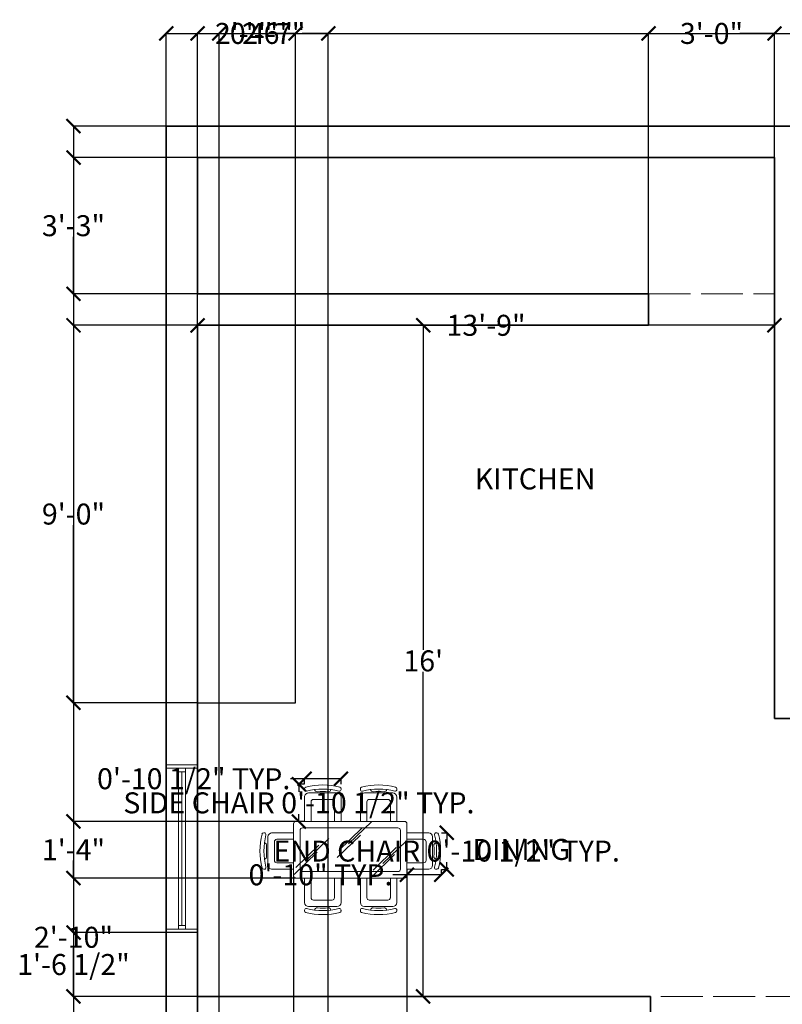
# Model space of a CAD drawing. Units: inches. Extents: x 43 to 543, y 36 to 629.
# Tile 4 of 5: x 43 to 261, y 348 to 629. Entities that reach past the tile are written whole.
import ezdxf

# ---------------------------------------------------------------- set-up
doc = ezdxf.new("R2010")
doc.units = ezdxf.units.IN
doc.header["$MEASUREMENT"] = 0
doc.linetypes.add('ACAD_ISO02W100', pattern=[15, 12, -3])
for name, color, linetype, lineweight in [('A-ANNO-DIMS', 2, 'Continuous', 18), ('A-AREA-IDEN', 7, 'Continuous', 25), ('A-FLOR-FIXT', 9, 'Continuous', 25), ('A-FURN', 8, 'Continuous', 13), ('A-GLAZ', 4, 'Continuous', 18), ('A-WALL', 7, 'Continuous', 35), ('A-WALL-OVHD', 7, 'ACAD_ISO02W100', 18)]:
    doc.layers.add(name, color=color, linetype=linetype, lineweight=lineweight)
doc.styles.get("Standard").update_dxf_attribs({"font": 'arial.ttf'})
doc.dimstyles.get("Standard").update_dxf_attribs({"dimtxt": 6, "dimasz": 4, "dimexe": 0.18, "dimexo": 0.0625, "dimgap": 0.09, "dimtad": 0, "dimtih": 1, "dimtoh": 1, "dimdec": 0, "dimzin": 0, "dimdsep": 46, "dimlunit": 4, "dimtxsty": 'Standard', "dimblk": 'ARCHTICK', "dimcen": 0.09, "dimadec": 0, "dimazin": 0, "dimtfac": 1, "dimtdec": 0, "dimtofl": 0, "dimtmove": 0, "dimatfit": 3, "dimldrblk": 'ARCHTICK', "dimfxl": 1, "dimtolj": 1, "dimtzin": 0, "dimarcsym": 1})

# ---------------------------------------------------------------- blocks, each defined once
blk = doc.blocks.new('TFHJBHN')
for p, q in [((347.02, 210.06), (338.02, 210.06)), ((347.02, 209.06), (338.02, 209.06)), ((341.52, 209.06), (341.52, 163.06)), ((343.52, 209.06), (343.52, 163.06)), ((343.52, 208.06), (341.52, 208.06)), ((342.52, 208.06), (342.52, 164.06)), ((341.52, 164.06), (343.52, 164.06)), ((338.02, 163.06), (347.02, 163.06)), ((338.02, 162.06), (347.02, 162.06))]:
    blk.add_line(p, q)
blk = doc.blocks.new('_ArchTick')
at = {"color": 0, "linetype": 'ByBlock', "const_width": 0.15}
blk.add_lwpolyline([(-0.5, -0.5), (0.5, 0.5)], dxfattribs=at)
blk = doc.blocks.new('*D8')
at = {"layer": 'A-ANNO-DIMS', "color": 0, "lineweight": -2, "transparency": 16777216}
for p, q in [((93.94, 542.02), (158.59, 542.02)), ((158.41, 542.02), (158.41, 449.17)), ((158.41, 350.02), (158.41, 442.86)), ((93.94, 350.02), (158.59, 350.02))]:
    blk.add_line(p, q, dxfattribs=at)
at = {"layer": 'Defpoints', "color": 0, "transparency": 16777216}
for p in [(93.88, 542.02), (158.41, 542.02), (93.88, 350.02)]:
    blk.add_point(p, dxfattribs=at)
at = {"layer": 'A-ANNO-DIMS', "color": 0, "lineweight": -2, "transparency": 16777216, "xscale": 4, "yscale": 4, "zscale": 4}
for p, rotation in [((158.41, 542.02), 90), ((158.41, 350.02), 270)]:
    blk.add_blockref('_ArchTick', p, dxfattribs=dict(at, rotation=rotation))
at = {"layer": 'A-ANNO-DIMS', "color": 0, "transparency": 16777216, "insert": (158.41, 446.02), "char_height": 6, "attachment_point": 5}
blk.add_mtext("\\A1;16'", dxfattribs=at)
blk = doc.blocks.new('*D9')
at = {"layer": 'A-ANNO-DIMS', "color": 0, "lineweight": -2, "transparency": 16777216}
for p, q in [((93.88, 542.08), (93.88, 542.2)), ((93.88, 542.02), (166.26, 542.02)), ((258.88, 542.02), (186.49, 542.02)), ((258.88, 541.95), (258.88, 541.84))]:
    blk.add_line(p, q, dxfattribs=at)
at = {"layer": 'Defpoints', "color": 0, "transparency": 16777216}
for p in [(93.88, 542.02), (93.88, 542.02), (258.88, 542.02)]:
    blk.add_point(p, dxfattribs=at)
at = {"layer": 'A-ANNO-DIMS', "color": 0, "lineweight": -2, "transparency": 16777216, "xscale": 4, "yscale": 4, "zscale": 4, "rotation": 180}
blk.add_blockref('_ArchTick', (93.88, 542.02), dxfattribs=at)
at = {"layer": 'A-ANNO-DIMS', "color": 0, "lineweight": -2, "transparency": 16777216, "xscale": 4, "yscale": 4, "zscale": 4}
blk.add_blockref('_ArchTick', (258.88, 542.02), dxfattribs=at)
at = {"layer": 'A-ANNO-DIMS', "color": 0, "transparency": 16777216, "insert": (176.38, 542.02), "char_height": 6, "attachment_point": 5}
blk.add_mtext('\\A1;13\'-9"', dxfattribs=at)
blk = doc.blocks.new('CHAIR-DINING')
for p, q in [((0, 10.43), (0, 3.44)), ((1.85, 10.43), (1.85, 4.83)), ((8.57, 4.83), (8.57, 10.43)), ((10.42, 3.44), (10.42, 10.43)), ((0, 3.57), (0, 3.34)), ((2.55, 4.14), (7.87, 4.14)), ((10.42, 3.34), (10.42, 3.57)), ((1.16, 2.28), (9.26, 2.28)), ((2.89, 1.3), (2.89, 1.23)), ((7.53, 1.3), (7.53, 1.23))]:
    blk.add_line(p, q)
for centre, radius, start, end in [((1.16, 3.44), 1.16, 180, 270), ((2.55, 4.83), 0.695, 180, 270), ((7.87, 4.83), 0.695, 270, 0), ((9.26, 3.44), 1.16, 270, 0), ((0.46, 1.29), 0.463, 75.6786, 185.9216), ((-0.69, 1.17), 0.695, 354.0784, 5.9216), ((0.46, 1.05), 0.463, 174.0784, 255.853), ((5.21, 19.88), 19.88, 255.853, 284.147), ((5.21, 19.88), 18.73, 255.6786, 284.3214), ((3.59, 1.23), 0.695, 85.0346, 173.9719), ((5.21, 19.88), 18.03, 265.0346, 274.9654), ((6.83, 1.23), 0.695, 6.0281, 94.9654), ((9.96, 1.29), 0.463, 354.0784, 104.3214), ((9.96, 1.05), 0.463, 284.147, 5.9216), ((11.11, 1.17), 0.695, 174.0784, 185.9216)]:
    blk.add_arc(centre, radius, start, end)
blk = doc.blocks.new('CHAIR-DINING-END')
for p, q in [((2.28, 9.26), (2.28, 1.16)), ((3.57, 10.42), (3.34, 10.42)), ((9.62, 10.42), (3.44, 10.42)), ((9.62, 8.57), (4.83, 8.57)), ((1.3, 7.53), (1.23, 7.53)), ((4.14, 7.87), (4.14, 2.55)), ((1.3, 2.89), (1.23, 2.89)), ((3.34, 0), (3.57, 0)), ((3.44, 0), (9.62, 0)), ((4.83, 1.85), (9.62, 1.85))]:
    blk.add_line(p, q)
for centre, radius, start, end in [((19.88, 5.21), 19.88, 165.853, 194.147), ((1.05, 9.96), 0.463, 84.0784, 165.853), ((1.17, 11.11), 0.695, 264.0784, 275.9216), ((19.88, 5.21), 18.73, 165.6786, 194.3214), ((1.29, 9.96), 0.463, 345.6786, 95.9216), ((3.44, 9.26), 1.16, 90, 180), ((4.83, 7.87), 0.695, 90, 180), ((1.23, 6.83), 0.695, 355.0346, 83.9719), ((19.88, 5.21), 18.03, 175.0346, 184.9654), ((1.23, 3.59), 0.695, 276.0281, 4.9654), ((1.05, 0.46), 0.463, 194.147, 275.9216), ((1.17, -0.69), 0.695, 84.0784, 95.9216), ((1.29, 0.46), 0.463, 264.0784, 14.3214), ((3.44, 1.16), 1.16, 180, 270), ((4.83, 2.55), 0.695, 180, 270)]:
    blk.add_arc(centre, radius, start, end)
blk = doc.blocks.new('*D31')
at = {"layer": 'A-ANNO-DIMS', "color": 0, "lineweight": -2, "transparency": 16777216}
for p, q in [((124.39, 410.71), (122.68, 410.71)), ((122.86, 410.71), (122.86, 408.59)), ((124.39, 400.08), (122.68, 400.08)), ((122.86, 400.08), (122.86, 402.2))]:
    blk.add_line(p, q, dxfattribs=at)
at = {"layer": 'Defpoints', "color": 0, "transparency": 16777216}
for p in [(124.45, 410.71), (122.86, 400.08), (124.45, 400.08)]:
    blk.add_point(p, dxfattribs=at)
at = {"layer": 'A-ANNO-DIMS', "color": 0, "lineweight": -2, "transparency": 16777216, "xscale": 4, "yscale": 4, "zscale": 4}
for p, rotation in [((122.86, 410.71), 90), ((122.86, 400.08), 270)]:
    blk.add_blockref('_ArchTick', p, dxfattribs=dict(at, rotation=rotation))
at = {"layer": 'A-ANNO-DIMS', "color": 0, "transparency": 16777216, "insert": (122.86, 405.4), "char_height": 6, "attachment_point": 5}
blk.add_mtext('\\A1;SIDE CHAIR 0\'-10 1/2" TYP.', dxfattribs=at)
blk = doc.blocks.new('*D32')
at = {"layer": 'A-ANNO-DIMS', "color": 0, "lineweight": -2, "transparency": 16777216}
for p, q in [((124.45, 412.3), (120.45, 412.3)), ((124.45, 410.77), (124.45, 412.48)), ((134.92, 412.3), (124.45, 412.3)), ((134.92, 410.77), (134.92, 412.48))]:
    blk.add_line(p, q, dxfattribs=at)
at = {"layer": 'Defpoints', "color": 0, "transparency": 16777216}
for p in [(124.45, 412.3), (124.45, 410.71), (134.92, 410.71)]:
    blk.add_point(p, dxfattribs=at)
at = {"layer": 'A-ANNO-DIMS', "color": 0, "lineweight": -2, "transparency": 16777216, "xscale": 4, "yscale": 4, "zscale": 4, "rotation": 180}
blk.add_blockref('_ArchTick', (124.45, 412.3), dxfattribs=at)
at = {"layer": 'A-ANNO-DIMS', "color": 0, "lineweight": -2, "transparency": 16777216, "xscale": 4, "yscale": 4, "zscale": 4}
blk.add_blockref('_ArchTick', (134.92, 412.3), dxfattribs=at)
at = {"layer": 'A-ANNO-DIMS', "color": 0, "transparency": 16777216, "insert": (92.76, 412.3), "char_height": 6, "attachment_point": 5}
blk.add_mtext('\\A1;0\'-10 1/2" TYP.', dxfattribs=at)
blk = doc.blocks.new('*D33')
at = {"layer": 'A-ANNO-DIMS', "color": 0, "lineweight": -2, "transparency": 16777216}
for p, q in [((163.63, 396.84), (165.32, 396.84)), ((165.14, 396.84), (165.14, 394.8)), ((163.63, 386.38), (165.32, 386.38)), ((165.14, 386.38), (165.14, 388.42))]:
    blk.add_line(p, q, dxfattribs=at)
at = {"layer": 'Defpoints', "color": 0, "transparency": 16777216}
for p in [(163.57, 396.84), (163.57, 386.38), (165.14, 386.38)]:
    blk.add_point(p, dxfattribs=at)
at = {"layer": 'A-ANNO-DIMS', "color": 0, "lineweight": -2, "transparency": 16777216, "xscale": 4, "yscale": 4, "zscale": 4}
for p, rotation in [((165.14, 396.84), 90), ((165.14, 386.38), 270)]:
    blk.add_blockref('_ArchTick', p, dxfattribs=dict(at, rotation=rotation))
at = {"layer": 'A-ANNO-DIMS', "color": 0, "transparency": 16777216, "insert": (165.14, 391.61), "char_height": 6, "attachment_point": 5}
blk.add_mtext('\\A1;END CHAIR 0\'-10 1/2" TYP.', dxfattribs=at)
blk = doc.blocks.new('*D34')
at = {"layer": 'A-ANNO-DIMS', "color": 0, "lineweight": -2, "transparency": 16777216}
for p, q in [((153.74, 386.32), (153.74, 384.63)), ((163.57, 386.32), (163.57, 384.63)), ((153.74, 384.81), (149.74, 384.81)), ((163.57, 384.81), (153.74, 384.81))]:
    blk.add_line(p, q, dxfattribs=at)
at = {"layer": 'Defpoints', "color": 0, "transparency": 16777216}
for p in [(153.74, 386.38), (163.57, 386.38), (153.74, 384.81)]:
    blk.add_point(p, dxfattribs=at)
at = {"layer": 'A-ANNO-DIMS', "color": 0, "lineweight": -2, "transparency": 16777216, "xscale": 4, "yscale": 4, "zscale": 4, "rotation": 180}
blk.add_blockref('_ArchTick', (153.74, 384.81), dxfattribs=at)
at = {"layer": 'A-ANNO-DIMS', "color": 0, "lineweight": -2, "transparency": 16777216, "xscale": 4, "yscale": 4, "zscale": 4}
blk.add_blockref('_ArchTick', (163.57, 384.81), dxfattribs=at)
at = {"layer": 'A-ANNO-DIMS', "color": 0, "transparency": 16777216, "insert": (129.04, 384.81), "char_height": 6, "attachment_point": 5}
blk.add_mtext('\\A1;0\'-10" TYP.', dxfattribs=at)
blk = doc.blocks.new('*D37')
at = {"layer": 'A-ANNO-DIMS', "color": 0, "lineweight": -2, "transparency": 16777216}
for p, q in [((84.88, 599.08), (84.88, 625.7)), ((84.88, 625.52), (266.48, 625.52)), ((468.88, 625.52), (287.27, 625.52)), ((468.88, 599.08), (468.88, 625.7))]:
    blk.add_line(p, q, dxfattribs=at)
at = {"layer": 'Defpoints', "color": 0, "transparency": 16777216}
for p in [(468.88, 625.52), (84.88, 599.02), (468.88, 599.02)]:
    blk.add_point(p, dxfattribs=at)
at = {"layer": 'A-ANNO-DIMS', "color": 0, "lineweight": -2, "transparency": 16777216, "xscale": 4, "yscale": 4, "zscale": 4, "rotation": 180}
blk.add_blockref('_ArchTick', (84.88, 625.52), dxfattribs=at)
at = {"layer": 'A-ANNO-DIMS', "color": 0, "lineweight": -2, "transparency": 16777216, "xscale": 4, "yscale": 4, "zscale": 4}
blk.add_blockref('_ArchTick', (468.88, 625.52), dxfattribs=at)
at = {"layer": 'A-ANNO-DIMS', "color": 0, "transparency": 16777216, "insert": (276.88, 625.52), "char_height": 6, "attachment_point": 5}
blk.add_mtext('\\A1;32\'-0"', dxfattribs=at)
blk = doc.blocks.new('*D38')
at = {"layer": 'A-ANNO-DIMS', "color": 0, "lineweight": -2, "transparency": 16777216}
for p, q in [((84.82, 599.02), (58.2, 599.02)), ((58.38, 599.02), (58.38, 338.17)), ((58.38, 71.02), (58.38, 331.86)), ((84.82, 71.02), (58.2, 71.02))]:
    blk.add_line(p, q, dxfattribs=at)
at = {"layer": 'Defpoints', "color": 0, "transparency": 16777216}
for p in [(58.38, 599.02), (84.88, 599.02), (84.88, 71.02)]:
    blk.add_point(p, dxfattribs=at)
at = {"layer": 'A-ANNO-DIMS', "color": 0, "lineweight": -2, "transparency": 16777216, "xscale": 4, "yscale": 4, "zscale": 4}
for p, rotation in [((58.38, 599.02), 90), ((58.38, 71.02), 270)]:
    blk.add_blockref('_ArchTick', p, dxfattribs=dict(at, rotation=rotation))
at = {"layer": 'A-ANNO-DIMS', "color": 0, "transparency": 16777216, "insert": (58.38, 335.02), "char_height": 6, "attachment_point": 5}
blk.add_mtext('\\A1;44\'-0"', dxfattribs=at)
blk = doc.blocks.new('*D41')
at = {"layer": 'A-ANNO-DIMS', "color": 0, "lineweight": -2, "transparency": 16777216}
for p, q in [((93.82, 368.28), (58.2, 368.28)), ((58.38, 368.28), (58.38, 362.34)), ((58.38, 350.02), (58.38, 355.96)), ((93.82, 350.02), (58.2, 350.02))]:
    blk.add_line(p, q, dxfattribs=at)
at = {"layer": 'Defpoints', "color": 0, "transparency": 16777216}
for p in [(58.38, 368.28), (93.88, 368.28), (93.88, 350.02)]:
    blk.add_point(p, dxfattribs=at)
at = {"layer": 'A-ANNO-DIMS', "color": 0, "lineweight": -2, "transparency": 16777216, "xscale": 4, "yscale": 4, "zscale": 4}
for p, rotation in [((58.38, 368.28), 90), ((58.38, 350.02), 270)]:
    blk.add_blockref('_ArchTick', p, dxfattribs=dict(at, rotation=rotation))
at = {"layer": 'A-ANNO-DIMS', "color": 0, "transparency": 16777216, "insert": (58.38, 359.15), "char_height": 6, "attachment_point": 5}
blk.add_mtext('\\A1;1\'-6 1/2"', dxfattribs=at)
blk = doc.blocks.new('*D44')
at = {"layer": 'A-ANNO-DIMS', "color": 0, "lineweight": -2, "transparency": 16777216}
for p, q in [((121.33, 384.5), (121.33, 44.34)), ((153.74, 384.5), (153.74, 44.34)), ((121.33, 44.52), (122.43, 44.52)), ((153.74, 44.52), (152.64, 44.52))]:
    blk.add_line(p, q, dxfattribs=at)
at = {"layer": 'Defpoints', "color": 0, "transparency": 16777216}
for p in [(121.33, 384.57), (153.74, 384.57), (153.74, 44.52)]:
    blk.add_point(p, dxfattribs=at)
at = {"layer": 'A-ANNO-DIMS', "color": 0, "lineweight": -2, "transparency": 16777216, "xscale": 4, "yscale": 4, "zscale": 4, "rotation": 180}
blk.add_blockref('_ArchTick', (121.33, 44.52), dxfattribs=at)
at = {"layer": 'A-ANNO-DIMS', "color": 0, "lineweight": -2, "transparency": 16777216, "xscale": 4, "yscale": 4, "zscale": 4}
blk.add_blockref('_ArchTick', (153.74, 44.52), dxfattribs=at)
at = {"layer": 'A-ANNO-DIMS', "color": 0, "transparency": 16777216, "insert": (137.54, 44.52), "char_height": 6, "attachment_point": 5}
blk.add_mtext('\\A1;2\'-8 1/2"', dxfattribs=at)
blk = doc.blocks.new('*D45')
at = {"layer": 'A-ANNO-DIMS', "color": 0, "lineweight": -2, "transparency": 16777216}
for p, q in [((121.96, 400.08), (58.2, 400.08)), ((58.38, 400.08), (58.38, 395.08)), ((58.38, 383.87), (58.38, 388.87)), ((121.96, 383.87), (58.2, 383.87))]:
    blk.add_line(p, q, dxfattribs=at)
at = {"layer": 'Defpoints', "color": 0, "transparency": 16777216}
for p in [(122.02, 400.08), (58.38, 383.87), (122.02, 383.87)]:
    blk.add_point(p, dxfattribs=at)
at = {"layer": 'A-ANNO-DIMS', "color": 0, "lineweight": -2, "transparency": 16777216, "xscale": 4, "yscale": 4, "zscale": 4}
for p, rotation in [((58.38, 400.08), 90), ((58.38, 383.87), 270)]:
    blk.add_blockref('_ArchTick', p, dxfattribs=dict(at, rotation=rotation))
at = {"layer": 'A-ANNO-DIMS', "color": 0, "transparency": 16777216, "insert": (58.38, 391.98), "char_height": 6, "attachment_point": 5}
blk.add_mtext('\\A1;1\'-4"', dxfattribs=at)
blk = doc.blocks.new('*D50')
at = {"layer": 'A-ANNO-DIMS', "color": 0, "lineweight": -2, "transparency": 16777216}
for p, q in [((93.88, 542.08), (93.88, 625.7)), ((93.88, 625.52), (99.76, 625.52)), ((121.88, 625.52), (115.99, 625.52)), ((121.88, 542.08), (121.88, 625.7))]:
    blk.add_line(p, q, dxfattribs=at)
at = {"layer": 'Defpoints', "color": 0, "transparency": 16777216}
for p in [(121.88, 625.52), (93.88, 542.02), (121.88, 542.02)]:
    blk.add_point(p, dxfattribs=at)
at = {"layer": 'A-ANNO-DIMS', "color": 0, "lineweight": -2, "transparency": 16777216, "xscale": 4, "yscale": 4, "zscale": 4, "rotation": 180}
blk.add_blockref('_ArchTick', (93.88, 625.52), dxfattribs=at)
at = {"layer": 'A-ANNO-DIMS', "color": 0, "lineweight": -2, "transparency": 16777216, "xscale": 4, "yscale": 4, "zscale": 4}
blk.add_blockref('_ArchTick', (121.88, 625.52), dxfattribs=at)
at = {"layer": 'A-ANNO-DIMS', "color": 0, "transparency": 16777216, "insert": (107.88, 625.52), "char_height": 6, "attachment_point": 5}
blk.add_mtext('\\A1;2\'-4"', dxfattribs=at)
blk = doc.blocks.new('*D51')
at = {"layer": 'A-ANNO-DIMS', "color": 0, "lineweight": -2, "transparency": 16777216}
for p, q in [((93.82, 542.02), (58.2, 542.02)), ((58.38, 542.02), (58.38, 491.17)), ((58.38, 434.02), (58.38, 484.86)), ((93.82, 434.02), (58.2, 434.02))]:
    blk.add_line(p, q, dxfattribs=at)
at = {"layer": 'Defpoints', "color": 0, "transparency": 16777216}
for p in [(58.38, 542.02), (93.88, 542.02), (93.88, 434.02)]:
    blk.add_point(p, dxfattribs=at)
at = {"layer": 'A-ANNO-DIMS', "color": 0, "lineweight": -2, "transparency": 16777216, "xscale": 4, "yscale": 4, "zscale": 4}
for p, rotation in [((58.38, 542.02), 90), ((58.38, 434.02), 270)]:
    blk.add_blockref('_ArchTick', p, dxfattribs=dict(at, rotation=rotation))
at = {"layer": 'A-ANNO-DIMS', "color": 0, "transparency": 16777216, "insert": (58.38, 488.02), "char_height": 6, "attachment_point": 5}
blk.add_mtext('\\A1;9\'-0"', dxfattribs=at)
blk = doc.blocks.new('*D52')
at = {"layer": 'A-ANNO-DIMS', "color": 0, "lineweight": -2, "transparency": 16777216}
for p, q in [((93.82, 590.02), (58.2, 590.02)), ((58.38, 590.02), (58.38, 573.67)), ((58.38, 551.02), (58.38, 567.36)), ((93.82, 551.02), (58.2, 551.02))]:
    blk.add_line(p, q, dxfattribs=at)
at = {"layer": 'Defpoints', "color": 0, "transparency": 16777216}
for p in [(58.38, 590.02), (93.88, 590.02), (93.88, 551.02)]:
    blk.add_point(p, dxfattribs=at)
at = {"layer": 'A-ANNO-DIMS', "color": 0, "lineweight": -2, "transparency": 16777216, "xscale": 4, "yscale": 4, "zscale": 4}
for p, rotation in [((58.38, 590.02), 90), ((58.38, 551.02), 270)]:
    blk.add_blockref('_ArchTick', p, dxfattribs=dict(at, rotation=rotation))
at = {"layer": 'A-ANNO-DIMS', "color": 0, "transparency": 16777216, "insert": (58.38, 570.52), "char_height": 6, "attachment_point": 5}
blk.add_mtext('\\A1;3\'-3"', dxfattribs=at)
blk = doc.blocks.new('*D53')
at = {"layer": 'A-ANNO-DIMS', "color": 0, "lineweight": -2, "transparency": 16777216}
for p, q in [((222.88, 551.08), (222.88, 625.7)), ((222.88, 625.52), (232.81, 625.52)), ((258.88, 625.52), (248.94, 625.52)), ((258.88, 551.08), (258.88, 625.7))]:
    blk.add_line(p, q, dxfattribs=at)
at = {"layer": 'Defpoints', "color": 0, "transparency": 16777216}
for p in [(258.88, 625.52), (222.88, 551.02), (258.88, 551.02)]:
    blk.add_point(p, dxfattribs=at)
at = {"layer": 'A-ANNO-DIMS', "color": 0, "lineweight": -2, "transparency": 16777216, "xscale": 4, "yscale": 4, "zscale": 4, "rotation": 180}
blk.add_blockref('_ArchTick', (222.88, 625.52), dxfattribs=at)
at = {"layer": 'A-ANNO-DIMS', "color": 0, "lineweight": -2, "transparency": 16777216, "xscale": 4, "yscale": 4, "zscale": 4}
blk.add_blockref('_ArchTick', (258.88, 625.52), dxfattribs=at)
at = {"layer": 'A-ANNO-DIMS', "color": 0, "transparency": 16777216, "insert": (240.88, 625.52), "char_height": 6, "attachment_point": 5}
blk.add_mtext('\\A1;3\'-0"', dxfattribs=at)
blk = doc.blocks.new('*D57')
at = {"layer": 'A-ANNO-DIMS', "color": 0, "lineweight": -2, "transparency": 16777216}
for p, q in [((100.07, 299.91), (100.07, 625.7)), ((100.07, 625.52), (107.55, 625.52)), ((131.25, 625.52), (123.78, 625.52)), ((131.25, 297.32), (131.25, 625.7))]:
    blk.add_line(p, q, dxfattribs=at)
at = {"layer": 'Defpoints', "color": 0, "transparency": 16777216}
for p in [(131.25, 625.52), (100.07, 299.85), (131.25, 297.26)]:
    blk.add_point(p, dxfattribs=at)
at = {"layer": 'A-ANNO-DIMS', "color": 0, "lineweight": -2, "transparency": 16777216, "xscale": 4, "yscale": 4, "zscale": 4, "rotation": 180}
blk.add_blockref('_ArchTick', (100.07, 625.52), dxfattribs=at)
at = {"layer": 'A-ANNO-DIMS', "color": 0, "lineweight": -2, "transparency": 16777216, "xscale": 4, "yscale": 4, "zscale": 4}
blk.add_blockref('_ArchTick', (131.25, 625.52), dxfattribs=at)
at = {"layer": 'A-ANNO-DIMS', "color": 0, "transparency": 16777216, "insert": (115.66, 625.52), "char_height": 6, "attachment_point": 5}
blk.add_mtext('\\A1;2\'-7"', dxfattribs=at)
blk = doc.blocks.new('*D58')
at = {"layer": 'A-ANNO-DIMS', "color": 0, "lineweight": -2, "transparency": 16777216}
for p, q in [((93.88, 345.58), (93.88, 625.7)), ((93.88, 625.52), (100.07, 625.52)), ((100.07, 299.91), (100.07, 625.7)), ((100.07, 625.52), (104.07, 625.52))]:
    blk.add_line(p, q, dxfattribs=at)
at = {"layer": 'Defpoints', "color": 0, "transparency": 16777216}
for p in [(100.07, 625.52), (93.88, 345.52), (100.07, 299.85)]:
    blk.add_point(p, dxfattribs=at)
at = {"layer": 'A-ANNO-DIMS', "color": 0, "lineweight": -2, "transparency": 16777216, "xscale": 4, "yscale": 4, "zscale": 4, "rotation": 180}
blk.add_blockref('_ArchTick', (93.88, 625.52), dxfattribs=at)
at = {"layer": 'A-ANNO-DIMS', "color": 0, "lineweight": -2, "transparency": 16777216, "xscale": 4, "yscale": 4, "zscale": 4}
blk.add_blockref('_ArchTick', (100.07, 625.52), dxfattribs=at)
at = {"layer": 'A-ANNO-DIMS', "color": 0, "transparency": 16777216, "insert": (112.13, 625.52), "char_height": 6, "attachment_point": 5}
blk.add_mtext('\\A1;0\'-6"', dxfattribs=at)
blk = doc.blocks.new('*D60')
at = {"layer": 'A-ANNO-DIMS', "color": 0, "lineweight": -2, "transparency": 16777216}
for p, q in [((121.33, 384.5), (121.33, 44.34)), ((93.88, 349.95), (93.88, 44.34)), ((93.88, 44.52), (121.33, 44.52)), ((121.33, 44.52), (125.33, 44.52))]:
    blk.add_line(p, q, dxfattribs=at)
at = {"layer": 'Defpoints', "color": 0, "transparency": 16777216}
for p in [(121.33, 384.57), (93.88, 350.02), (121.33, 44.52)]:
    blk.add_point(p, dxfattribs=at)
at = {"layer": 'A-ANNO-DIMS', "color": 0, "lineweight": -2, "transparency": 16777216, "xscale": 4, "yscale": 4, "zscale": 4, "rotation": 180}
blk.add_blockref('_ArchTick', (93.88, 44.52), dxfattribs=at)
at = {"layer": 'A-ANNO-DIMS', "color": 0, "lineweight": -2, "transparency": 16777216, "xscale": 4, "yscale": 4, "zscale": 4}
blk.add_blockref('_ArchTick', (121.33, 44.52), dxfattribs=at)
at = {"layer": 'A-ANNO-DIMS', "color": 0, "transparency": 16777216, "insert": (140.43, 44.52), "char_height": 6, "attachment_point": 5}
blk.add_mtext('\\A1;2\'-3 1/2"', dxfattribs=at)
blk = doc.blocks.new('*D61')
at = {"layer": 'A-ANNO-DIMS', "color": 0, "lineweight": -2, "transparency": 16777216}
for p, q in [((121.96, 383.87), (58.2, 383.87)), ((58.38, 383.87), (58.38, 370.1)), ((58.38, 350.02), (58.38, 363.79)), ((93.82, 350.02), (58.2, 350.02))]:
    blk.add_line(p, q, dxfattribs=at)
at = {"layer": 'Defpoints', "color": 0, "transparency": 16777216}
for p in [(58.38, 383.87), (122.02, 383.87), (93.88, 350.02)]:
    blk.add_point(p, dxfattribs=at)
at = {"layer": 'A-ANNO-DIMS', "color": 0, "lineweight": -2, "transparency": 16777216, "xscale": 4, "yscale": 4, "zscale": 4}
for p, rotation in [((58.38, 383.87), 90), ((58.38, 350.02), 270)]:
    blk.add_blockref('_ArchTick', p, dxfattribs=dict(at, rotation=rotation))
at = {"layer": 'A-ANNO-DIMS', "color": 0, "transparency": 16777216, "insert": (58.38, 366.94), "char_height": 6, "attachment_point": 5}
blk.add_mtext('\\A1;2\'-10"', dxfattribs=at)

msp = doc.modelspace()

# ---------------------------------------------------------------- linework, layer by layer
at = {"layer": 'A-FLOR-FIXT'}
for p, q in [((121.88, 434.02), (121.88, 542.02)), ((93.88, 434.02), (121.88, 434.02))]:
    msp.add_line(p, q, dxfattribs=at)
at = {"layer": 'A-FURN'}
for p, q in [((153.05, 400.08), (122.02, 400.08)), ((137.09, 393.64), (143.72, 400.05)), ((121.33, 399.39), (121.33, 384.57)), ((123.18, 397.53), (123.18, 386.42)), ((151.2, 398.23), (123.87, 398.23)), ((134.27, 391.77), (140.9, 398.19)), ((151.89, 386.42), (151.89, 397.53)), ((153.74, 384.57), (153.74, 399.39)), ((124.76, 388.75), (131.38, 395.16)), ((133.81, 389.77), (140.44, 396.19)), ((146.87, 388.03), (153.5, 394.45)), ((121.94, 386.88), (128.56, 393.3)), ((144.06, 386.17), (150.68, 392.59)), ((121.48, 384.88), (128.1, 391.3)), ((143.6, 384.17), (150.22, 390.59)), ((122.02, 383.87), (153.05, 383.87)), ((123.87, 385.72), (151.2, 385.72))]:
    msp.add_line(p, q, dxfattribs=at)
for centre, start, end in [((122.02, 399.39), 90, 180), ((153.05, 399.39), 0, 90), ((123.87, 397.53), 90, 180), ((151.2, 397.53), 0, 90), ((123.87, 386.42), 180, 270), ((151.2, 386.42), 270, 0), ((122.02, 384.57), 180, 270), ((153.05, 384.57), 270, 0)]:
    msp.add_arc(centre, 0.695, start, end, dxfattribs=at)
at = {"layer": 'A-WALL'}
for p, q in [((84.88, 599.02), (468.88, 599.02)), ((84.88, 71.02), (84.88, 599.02)), ((93.88, 590.02), (258.88, 590.02)), ((93.88, 551.02), (93.88, 590.02)), ((258.88, 590.02), (258.88, 551.02)), ((93.88, 551.02), (222.88, 551.02)), ((222.88, 551.02), (222.88, 542.02)), ((258.88, 551.02), (258.88, 542.02)), ((93.88, 542.02), (222.88, 542.02)), ((93.88, 350.02), (93.88, 542.02)), ((258.88, 542.02), (258.88, 429.52)), ((258.88, 429.52), (263.38, 429.52)), ((93.88, 350.02), (223.38, 350.02)), ((223.38, 350.02), (223.38, 345.52))]:
    msp.add_line(p, q, dxfattribs=at)
at = {"layer": 'A-WALL-OVHD'}
for p, q in [((222.88, 551.02), (258.88, 551.02)), ((258.88, 551.02), (258.88, 542.02)), ((258.88, 542.02), (222.88, 542.02)), ((283.38, 350.02), (223.38, 350.02)), ((223.38, 350.02), (223.38, 345.52))]:
    msp.add_line(p, q, dxfattribs=at)

# ---------------------------------------------------------------- block references
at = {"layer": 'A-FURN', "rotation": 180}
for name, p in [('CHAIR-DINING', (134.9, 410.51)), ('CHAIR-DINING', (150.86, 410.51)), ('CHAIR-DINING-END', (163.37, 396.82))]:
    msp.add_blockref(name, p, dxfattribs=at)
at = {"layer": 'A-FURN'}
for name, p in [('CHAIR-DINING-END', (111.7, 386.4)), ('CHAIR-DINING', (124.48, 373.44)), ('CHAIR-DINING', (140.44, 373.44))]:
    msp.add_blockref(name, p, dxfattribs=at)
at = {"layer": 'A-GLAZ'}
msp.add_blockref('TFHJBHN', (-253.14, 206.22), dxfattribs=at)

# ---------------------------------------------------------------- texts
at = {"layer": 'A-AREA-IDEN', "char_height": 6, "attachment_point": 1}
for s, width, insert in [('\\pxqc;KITCHEN', 95.8575, (142.48, 501.08)), ('DINING', 58.0298, (172.52, 395.08))]:
    msp.add_mtext_dynamic_manual_height_columns(s, width=width, gutter_width=30, heights=[0], dxfattribs=dict(at, insert=insert))

# ---------------------------------------------------------------- dimensions: what is measured, and where the dimension line sits
at = {"layer": 'A-ANNO-DIMS'}
for base, p1, p2, override, picture, middle in [((468.88, 625.52), (84.88, 599.02), (468.88, 599.02), {"dimdec": 1, "dimlfac": 1, "dimrnd": 0, "dimzin": 1, "dimdsep": 46, "dimlunit": 4, "dimfrac": 2}, '*D37', (276.88, 625.52)), ((121.88, 625.52), (93.88, 542.02), (121.88, 542.02), {"dimdec": 1, "dimlfac": 1, "dimrnd": 0, "dimzin": 1, "dimdsep": 46, "dimlunit": 4, "dimfrac": 2}, '*D50', (107.88, 625.52)), ((100.07, 625.52), (93.88, 345.52), (100.07, 299.85), {"dimdec": 1, "dimlfac": 1, "dimrnd": 0, "dimzin": 1, "dimdsep": 46, "dimlunit": 4, "dimfrac": 2}, '*D58', (112.13, 625.52)), ((131.25, 625.52), (100.07, 299.85), (131.25, 297.26), {"dimdec": 1, "dimlfac": 1, "dimrnd": 0, "dimzin": 1, "dimdsep": 46, "dimlunit": 4, "dimfrac": 2}, '*D57', (115.66, 625.52)), ((258.88, 625.52), (222.88, 551.02), (258.88, 551.02), {"dimdec": 1, "dimlfac": 1, "dimrnd": 0, "dimzin": 1, "dimdsep": 46, "dimlunit": 4, "dimfrac": 2}, '*D53', (240.88, 625.52)), ((93.88, 542.02), (258.88, 542.02), (93.88, 542.02), {"dimclrd": 0, "dimclre": 0, "dimclrt": 0}, '*D9', (176.38, 542.02)), ((121.3278, 44.5166), (93.8776, 350.0166), (121.3278, 384.566), {"dimdec": 1, "dimlfac": 1, "dimrnd": 0, "dimzin": 1, "dimdsep": 46, "dimlunit": 4, "dimfrac": 2}, '*D60', (140.4341, 44.5166)), ((153.74, 44.52), (121.33, 384.57), (153.74, 384.57), {"dimdec": 1, "dimlfac": 1, "dimrnd": 0, "dimzin": 1, "dimdsep": 46, "dimlunit": 4, "dimfrac": 2}, '*D44', (137.54, 44.52))]:
    dim = msp.add_linear_dim(base=base, p1=p1, p2=p2, dimstyle='Standard', override=override, dxfattribs=at)
    dim.commit()
    dim.dimension.update_dxf_attribs({"geometry": picture, "text_midpoint": middle})
for base, p1, p2, override, picture, middle in [((58.38, 599.02), (84.88, 71.02), (84.88, 599.02), {"dimdec": 1, "dimlfac": 1, "dimrnd": 0, "dimzin": 1, "dimdsep": 46, "dimlunit": 4, "dimfrac": 2}, '*D38', (58.38, 335.02)), ((58.38, 590.02), (93.88, 551.02), (93.88, 590.02), {"dimdec": 1, "dimlfac": 1, "dimrnd": 0, "dimzin": 1, "dimdsep": 46, "dimlunit": 4, "dimfrac": 2}, '*D52', (58.38, 570.52)), ((58.38, 542.02), (93.88, 434.02), (93.88, 542.02), {"dimdec": 1, "dimlfac": 1, "dimrnd": 0, "dimzin": 1, "dimdsep": 46, "dimlunit": 4, "dimfrac": 2}, '*D51', (58.38, 488.02)), ((158.41, 542.02), (93.88, 350.02), (93.88, 542.02), {"dimclrd": 0, "dimclre": 0, "dimclrt": 0}, '*D8', (158.41, 446.02)), ((58.38, 383.87), (122.02, 400.08), (122.02, 383.87), {"dimdec": 1, "dimlfac": 1, "dimrnd": 0, "dimzin": 1, "dimdsep": 46, "dimlunit": 4, "dimfrac": 2}, '*D45', (58.38, 391.98)), ((58.3776, 383.8713), (93.8776, 350.0166), (122.0224, 383.8713), {"dimdec": 1, "dimlfac": 1, "dimrnd": 0, "dimzin": 1, "dimdsep": 46, "dimlunit": 4, "dimfrac": 2}, '*D61', (58.3776, 366.9439)), ((58.38, 368.28), (93.88, 350.02), (93.88, 368.28), {"dimdec": 1, "dimlfac": 1, "dimrnd": 0, "dimzin": 1, "dimdsep": 46, "dimlunit": 4, "dimfrac": 2}, '*D41', (58.38, 359.15))]:
    dim = msp.add_linear_dim(base=base, p1=p1, p2=p2, angle=90, dimstyle='Standard', override=override, dxfattribs=at)
    dim.commit()
    dim.dimension.update_dxf_attribs({"geometry": picture, "text_midpoint": middle})
for base, p1, p2, angle, text, picture, middle in [((122.86, 400.08), (124.45, 410.71), (124.45, 400.08), 270, 'SIDE CHAIR <> TYP.', '*D31', (122.86, 405.4)), ((124.45, 412.3), (134.92, 410.71), (124.45, 410.71), 180, '<> TYP.', '*D32', (92.76, 412.3)), ((165.14, 386.38), (163.57, 396.84), (163.57, 386.38), 270, 'END CHAIR <> TYP.', '*D33', (165.14, 391.61)), ((153.74, 384.81), (163.57, 386.38), (153.74, 386.38), 180, '<> TYP.', '*D34', (129.04, 384.81))]:
    dim = msp.add_linear_dim(base=base, p1=p1, p2=p2, angle=angle, text=text, dimstyle='Standard', override={"dimdec": 1, "dimlfac": 1, "dimrnd": 0, "dimzin": 1, "dimdsep": 46, "dimlunit": 4, "dimfrac": 2}, dxfattribs=at)
    dim.commit()
    dim.dimension.update_dxf_attribs({"geometry": picture, "text_midpoint": middle})

doc.saveas('drawing.dxf')
